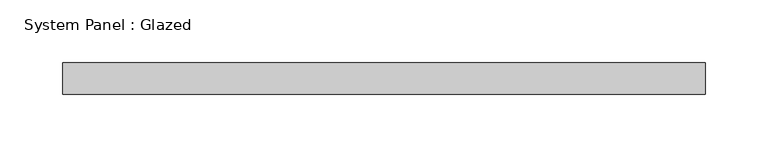
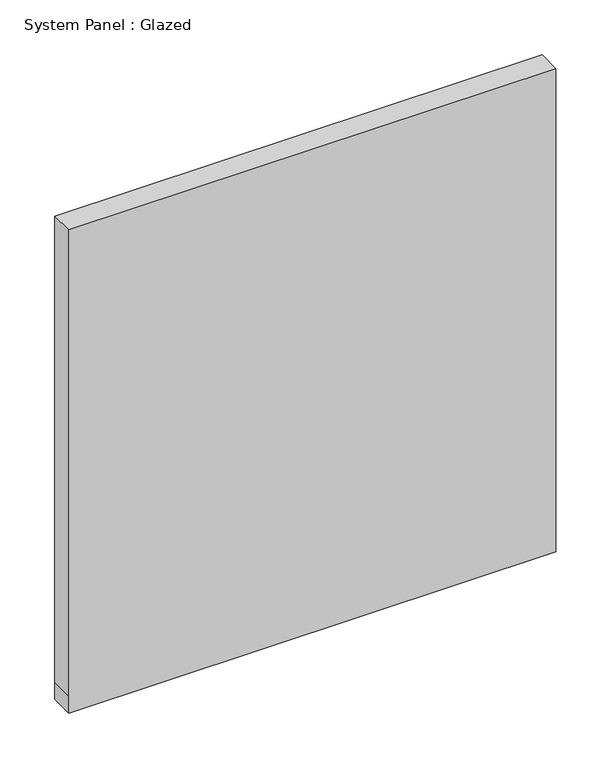
"""IFC4 building model written with IfcOpenShell, lengths in millimetres: plate geometry, System Panel : Glazed."""

from ifc_helpers import new_model, si_unit, frame, origin, place, context, project, spatial, polyline, outline, extrude, source, transform, mapped, element, save


def system_panel_glazed_83ea90e8(model_context):
    return source(origin(), model_context, "Body", "SweptSolid", [
        extrude(outline(polyline([(0.0, -257.175), (0.0, 257.175), (19.05, 257.175), (539.4467564, 257.175), (539.4467564, -257.175), (19.05, -257.175), (0.0, -257.175)])), frame((0.0, 19.05, 0.0), z_axis=(0.0, 1.0, 0.0), x_axis=(0.0, 0.0, 1.0)), (0.0, 0.0, 1.0), 25.4),
    ])


if __name__ == "__main__":
    model = new_model("IFC4")
    model_context = context("Model", 3, world=origin())
    ifc_project = project(units=[si_unit("LENGTHUNIT", "METRE", prefix="MILLI")], contexts=[model_context])
    site = spatial("IfcSite", under=ifc_project)
    building = spatial("IfcBuilding", under=site)
    placement = place(None, origin())
    system_panel_glazed_shape = system_panel_glazed_83ea90e8(model_context)
    element("IfcPlate", 1, ObjectType="System Panel : Glazed", at=placement, inside=building, context=model_context, shape_type="MappedRepresentation", body=[
        mapped(system_panel_glazed_shape, transform((0.0, 0.0, 0.0), x_axis=(1.0, 0.0, 0.0), y_axis=(0.0, 1.0, 0.0), z_axis=(0.0, 0.0, 1.0))),
    ])
    save(model, "model.ifc")

# Revit data of these elements
# Type "System Panel : Glazed"
#   Construction Type Id = "GSP4R"
#   Analytic Construction = "1/8 in Pilkington single glazing"
#   Visual Light Transmittance = 0.9
#   Solar Heat Gain Coefficient = 0.86
#   Heat Transfer Coefficient (U) = 1.18115 BTU/(h·ft²·°F)
#   Define Thermal Properties by = 1
# Element 1 (IfcPlate, "System Panel : Glazed")
#   Materials on its faces: "Glass"
# Materials
#   "Glass": class "Glass", colour RGB 0 128 192, transparency 0.75, Description = "Soda Lime Glass", Cost = 0
